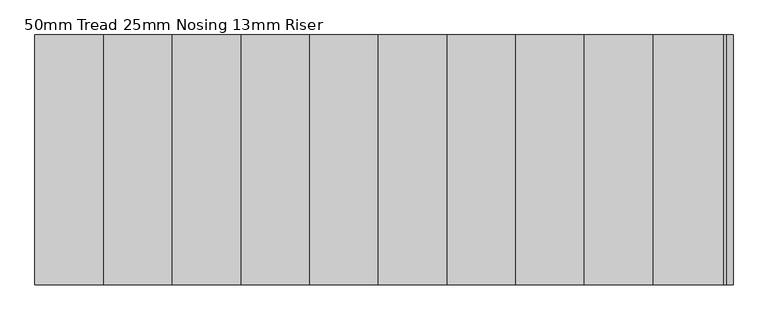
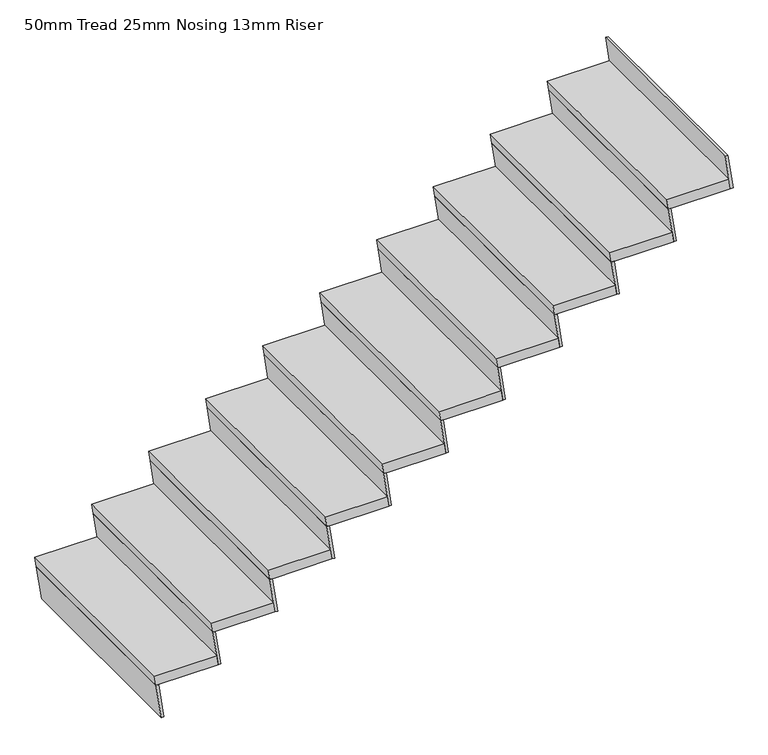
"""IFC4 building model written with IfcOpenShell, lengths in millimetres: stair flight geometry, 50mm Tread 25mm Nosing 13mm Riser."""

from ifc_helpers import new_model, si_unit, frame, origin, place, context, project, spatial, polyline, outline, extrude, source, transform, mapped, element, save


def stair_flight_50mm_tread_25mm_nosing_13mm_riser_b2cb06da(model_context):
    return source(origin(), model_context, "Body", "SweptSolid", [
        extrude(outline(polyline([(1739.1304348, -10174.8492596), (1739.1304348, -10474.8492596), (1689.1304348, -10467.6617596), (1689.1304348, -10167.6617596), (1739.1304348, -10174.8492596)])), frame((0.0, 3570.530447, 0.0), z_axis=(0.0, 1.0, 0.0), x_axis=(0.0, 0.0, 1.0)), (0.0, 0.0, 1.0), 1000.0257812),
        extrude(outline(polyline([(1689.1304348, -10467.6617596), (1515.2173913, -10442.6617596), (1515.2173913, -10430.0332696), (1689.1304348, -10455.0332696), (1689.1304348, -10467.6617596)])), frame((0.0, 3570.530447, 0.0), z_axis=(0.0, 1.0, 0.0), x_axis=(0.0, 0.0, 1.0)), (0.0, 0.0, 1.0), 1000.0257813),
        extrude(outline(polyline([(1863.0434783, -10192.6617596), (1689.1304348, -10167.6617596), (1689.1304348, -10155.0332696), (1863.0434783, -10180.0332696), (1863.0434783, -10192.6617596)])), frame((0.0, 3570.530447, 0.0), z_axis=(0.0, 1.0, 0.0), x_axis=(0.0, 0.0, 1.0)), (0.0, 0.0, 1.0), 1000.0257813),
        extrude(outline(polyline([(1913.0434783, -9899.8492596), (1913.0434783, -10199.8492596), (1863.0434783, -10192.6617596), (1863.0434783, -9892.6617596), (1913.0434783, -9899.8492596)])), frame((0.0, 3570.530447, 0.0), z_axis=(0.0, 1.0, 0.0), x_axis=(0.0, 0.0, 1.0)), (0.0, 0.0, 1.0), 1000.0257813),
        extrude(outline(polyline([(2036.9565217, -9917.6617596), (1863.0434783, -9892.6617596), (1863.0434783, -9880.0332696), (2036.9565217, -9905.0332696), (2036.9565217, -9917.6617596)])), frame((0.0, 3570.530447, 0.0), z_axis=(0.0, 1.0, 0.0), x_axis=(0.0, 0.0, 1.0)), (0.0, 0.0, 1.0), 1000.0257813),
        extrude(outline(polyline([(2086.9565217, -9624.8492596), (2086.9565217, -9924.8492596), (2036.9565217, -9917.6617596), (2036.9565217, -9617.6617596), (2086.9565217, -9624.8492596)])), frame((0.0, 3570.530447, 0.0), z_axis=(0.0, 1.0, 0.0), x_axis=(0.0, 0.0, 1.0)), (0.0, 0.0, 1.0), 1000.0257813),
        extrude(outline(polyline([(2210.8695652, -9642.6617596), (2036.9565217, -9617.6617596), (2036.9565217, -9605.0332696), (2210.8695652, -9630.0332696), (2210.8695652, -9642.6617596)])), frame((0.0, 3570.530447, 0.0), z_axis=(0.0, 1.0, 0.0), x_axis=(0.0, 0.0, 1.0)), (0.0, 0.0, 1.0), 1000.0257813),
        extrude(outline(polyline([(2260.8695652, -9349.8492596), (2260.8695652, -9649.8492596), (2210.8695652, -9642.6617596), (2210.8695652, -9342.6617596), (2260.8695652, -9349.8492596)])), frame((0.0, 3570.530447, 0.0), z_axis=(0.0, 1.0, 0.0), x_axis=(0.0, 0.0, 1.0)), (0.0, 0.0, 1.0), 1000.0257812),
        extrude(outline(polyline([(2384.7826087, -9367.6617596), (2210.8695652, -9342.6617596), (2210.8695652, -9330.0332696), (2384.7826087, -9355.0332696), (2384.7826087, -9367.6617596)])), frame((0.0, 3570.530447, 0.0), z_axis=(0.0, 1.0, 0.0), x_axis=(0.0, 0.0, 1.0)), (0.0, 0.0, 1.0), 1000.0257813),
        extrude(outline(polyline([(2434.7826087, -9074.8492596), (2434.7826087, -9374.8492596), (2384.7826087, -9367.6617596), (2384.7826087, -9067.6617596), (2434.7826087, -9074.8492596)])), frame((0.0, 3570.530447, 0.0), z_axis=(0.0, 1.0, 0.0), x_axis=(0.0, 0.0, 1.0)), (0.0, 0.0, 1.0), 1000.0257813),
        extrude(outline(polyline([(2558.6956522, -9092.6617596), (2384.7826087, -9067.6617596), (2384.7826087, -9055.0332696), (2558.6956522, -9080.0332696), (2558.6956522, -9092.6617596)])), frame((0.0, 3570.530447, 0.0), z_axis=(0.0, 1.0, 0.0), x_axis=(0.0, 0.0, 1.0)), (0.0, 0.0, 1.0), 1000.0257813),
        extrude(outline(polyline([(2608.6956522, -8799.8492596), (2608.6956522, -9099.8492596), (2558.6956522, -9092.6617596), (2558.6956522, -8792.6617596), (2608.6956522, -8799.8492596)])), frame((0.0, 3570.530447, 0.0), z_axis=(0.0, 1.0, 0.0), x_axis=(0.0, 0.0, 1.0)), (0.0, 0.0, 1.0), 1000.0257813),
        extrude(outline(polyline([(2732.6086957, -8817.6617596), (2558.6956522, -8792.6617596), (2558.6956522, -8780.0332696), (2732.6086957, -8805.0332696), (2732.6086957, -8817.6617596)])), frame((0.0, 3570.530447, 0.0), z_axis=(0.0, 1.0, 0.0), x_axis=(0.0, 0.0, 1.0)), (0.0, 0.0, 1.0), 1000.0257812),
        extrude(outline(polyline([(2782.6086957, -8524.8492596), (2782.6086957, -8824.8492596), (2732.6086957, -8817.6617596), (2732.6086957, -8517.6617596), (2782.6086957, -8524.8492596)])), frame((0.0, 3570.530447, 0.0), z_axis=(0.0, 1.0, 0.0), x_axis=(0.0, 0.0, 1.0)), (0.0, 0.0, 1.0), 1000.0257812),
        extrude(outline(polyline([(2906.5217391, -8542.6617596), (2732.6086957, -8517.6617596), (2732.6086957, -8505.0332696), (2906.5217391, -8530.0332696), (2906.5217391, -8542.6617596)])), frame((0.0, 3570.530447, 0.0), z_axis=(0.0, 1.0, 0.0), x_axis=(0.0, 0.0, 1.0)), (0.0, 0.0, 1.0), 1000.0257813),
        extrude(outline(polyline([(2956.5217391, -8249.8492596), (2956.5217391, -8549.8492596), (2906.5217391, -8542.6617596), (2906.5217391, -8242.6617596), (2956.5217391, -8249.8492596)])), frame((0.0, 3570.530447, 0.0), z_axis=(0.0, 1.0, 0.0), x_axis=(0.0, 0.0, 1.0)), (0.0, 0.0, 1.0), 1000.0257813),
        extrude(outline(polyline([(3080.4347826, -8267.6617596), (2906.5217391, -8242.6617596), (2906.5217391, -8230.0332696), (3080.4347826, -8255.0332696), (3080.4347826, -8267.6617596)])), frame((0.0, 3570.530447, 0.0), z_axis=(0.0, 1.0, 0.0), x_axis=(0.0, 0.0, 1.0)), (0.0, 0.0, 1.0), 1000.0257813),
        extrude(outline(polyline([(3130.4347826, -7974.8492596), (3130.4347826, -8274.8492596), (3080.4347826, -8267.6617596), (3080.4347826, -7967.6617596), (3130.4347826, -7974.8492596)])), frame((0.0, 3570.530447, 0.0), z_axis=(0.0, 1.0, 0.0), x_axis=(0.0, 0.0, 1.0)), (0.0, 0.0, 1.0), 1000.0257813),
        extrude(outline(polyline([(3254.3478261, -7992.6617596), (3080.4347826, -7967.6617596), (3080.4347826, -7955.0332696), (3254.3478261, -7980.0332696), (3254.3478261, -7992.6617596)])), frame((0.0, 3570.530447, 0.0), z_axis=(0.0, 1.0, 0.0), x_axis=(0.0, 0.0, 1.0)), (0.0, 0.0, 1.0), 1000.0257812),
        extrude(outline(polyline([(3428.2608696, -7717.6617596), (3254.3478261, -7692.6617596), (3254.3478261, -7680.0332696), (3428.2608696, -7705.0332696), (3428.2608696, -7717.6617596)])), frame((0.0, 3570.530447, 0.0), z_axis=(0.0, 1.0, 0.0), x_axis=(0.0, 0.0, 1.0)), (0.0, 0.0, 1.0), 1000.0257813),
        extrude(outline(polyline([(3304.3478261, -7699.8492596), (3304.3478261, -7999.8492596), (3254.3478261, -7992.6617596), (3254.3478261, -7692.6617596), (3304.3478261, -7699.8492596)])), frame((0.0, 3570.530447, 0.0), z_axis=(0.0, 1.0, 0.0), x_axis=(0.0, 0.0, 1.0)), (0.0, 0.0, 1.0), 1000.0257812),
    ])


if __name__ == "__main__":
    model = new_model("IFC4")
    model_context = context("Model", 3, world=origin())
    ifc_project = project(units=[si_unit("LENGTHUNIT", "METRE", prefix="MILLI")], contexts=[model_context])
    site = spatial("IfcSite", under=ifc_project)
    building = spatial("IfcBuilding", under=site)
    placement = place(None, origin())
    stair_flight_50mm_tread_25mm_nosing_13mm_riser_shape = stair_flight_50mm_tread_25mm_nosing_13mm_riser_b2cb06da(model_context)
    element("IfcStairFlight", 1, ObjectType="50mm Tread 25mm Nosing 13mm Riser", at=placement, inside=building, context=model_context, shape_type="MappedRepresentation", body=[
        mapped(stair_flight_50mm_tread_25mm_nosing_13mm_riser_shape, transform((0.0, 0.0, 0.0), x_axis=(1.0, 0.0, 0.0), y_axis=(0.0, 1.0, 0.0), z_axis=(0.0, 0.0, 1.0))),
    ])
    save(model, "model.ifc")
